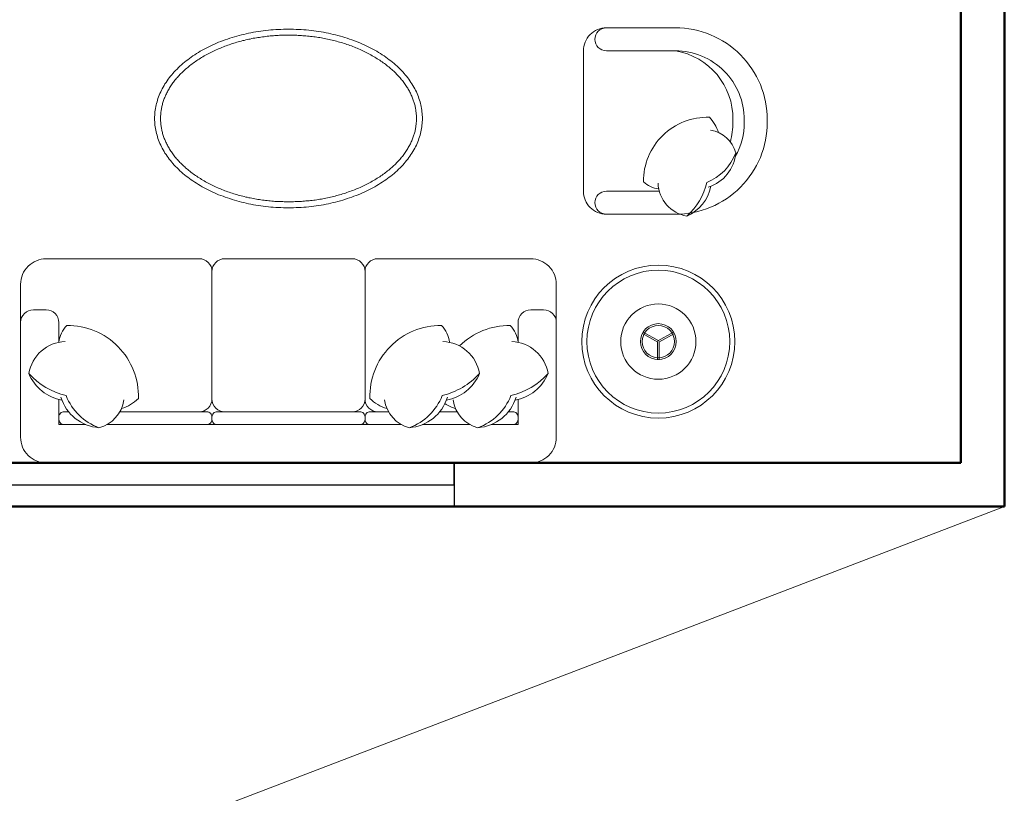
# Model space of a CAD drawing. Units: inches. Extents: x 1901 to 2863, y 888 to 2433.
# Tile 68 of 91: x 2651 to 2753, y 1732 to 1812. Entities that reach past the tile are written whole.
import ezdxf

# ---------------------------------------------------------------- set-up
doc = ezdxf.new("R2010")
doc.units = ezdxf.units.IN
for name, color, linetype, lineweight in [('A-ANNO-SYMB', 8, 'Continuous', 13), ('A-FURN', 8, 'Continuous', 18), ('A-GLAZ', 3, 'Continuous', 25), ('A-WALL', 7, 'Continuous', 50)]:
    doc.layers.add(name, color=color, linetype=linetype, lineweight=lineweight)

# ---------------------------------------------------------------- blocks, each defined once
blk = doc.blocks.new('WIN-60')
for p, q in [((0, 4.5), (0, 0)), ((60, 2.25), (60, 4.5)), ((60, 4.5), (60, 0)), ((0, 0), (0, 2.25)), ((0, 2.25), (60, 2.25))]:
    blk.add_line(p, q)

msp = doc.modelspace()

# ---------------------------------------------------------------- linework, layer by layer
at = {"layer": 'A-ANNO-SYMB'}
msp.add_line((2752.93, 1761.63), (2502.24, 1665.63), dxfattribs=at)
at = {"layer": 'A-FURN', "ltscale": 0.03}
for p, q in [((2717.24, 1778.55), (2715.64, 1779.47)), ((2717.32, 1778.69), (2715.72, 1779.61)), ((2717.24, 1778.69), (2718.85, 1779.61)), ((2717.32, 1778.55), (2718.93, 1779.47)), ((2717.2, 1778.62), (2717.2, 1776.76)), ((2717.36, 1778.62), (2717.36, 1776.76))]:
    msp.add_line(p, q, dxfattribs=at)
msp.add_lwpolyline([(2709.56, 1801.35), (2709.56, 1808.58, -0.414214), (2711.93, 1810.95), (2719.04, 1810.95, -0.414214), (2728.51, 1801.47), (2728.51, 1801.35), (2728.51, 1801.23, -0.414214), (2719.04, 1791.75), (2711.93, 1791.75, -0.414214), (2709.56, 1794.12), (2709.56, 1801.35)], format="xyb", dxfattribs=at)
at = {"layer": 'A-FURN'}
for points in [[(2719.04, 1808.58), (2711.93, 1808.58, -0.414214), (2710.74, 1809.76), (2710.74, 1809.76, -0.414214), (2711.93, 1810.95)], [(2719.04, 1808.58, -0.372719), (2724.96, 1801.47), (2724.96, 1801.35)], [(2719.04, 1808.58, -0.414214), (2726.14, 1801.47), (2726.14, 1801.35)], [(2717.32, 1794.36, -0.165541), (2715.75, 1795.09, -0.425989), (2722.54, 1801.74, -0.121523), (2723.47, 1800.16, 7.115464)], [(2724.7, 1799.21, 0.072384), (2724.96, 1801.23), (2724.96, 1801.35)], [(2725.21, 1797.7, 0.130591), (2726.14, 1801.23), (2726.14, 1801.35)], [(2722.43, 1794.54, 0.306663), (2725.25, 1798.08, 0.30633), (2722.67, 1800.39, -0.872847)], [(2720.23, 1791.56, 0.14773), (2722.27, 1795.02, 0.213343), (2725.25, 1798.08, 0.178662)], [(2717.25, 1794.95, 0.356772), (2720.23, 1791.56, 0.249542), (2722.69, 1794.63, -9.61688)], [(2717.37, 1794.12), (2711.93, 1794.12, 0.414214), (2710.74, 1792.94), (2710.74, 1792.94, 0.414214), (2711.93, 1791.75)], [(2669.98, 1771.39, 0.414214), (2671.29, 1772.7), (2671.29, 1785.84, 0.414214)], [(2688.37, 1771.39, -0.414214), (2687.06, 1772.7), (2687.06, 1785.84, -0.414214)], [(2651.58, 1780.59, -0.414214), (2652.9, 1781.9), (2654.21, 1781.9, -0.414214), (2655.52, 1780.59), (2655.52, 1778.55)], [(2702.83, 1778.55), (2702.83, 1780.59, -0.414214), (2704.14, 1781.9), (2705.46, 1781.9, -0.414214), (2706.77, 1780.59)], [(2655.52, 1778.55, -0.165541), (2656.33, 1780.29, -0.425989), (2663.71, 1772.76, -0.121523), (2661.96, 1771.72, 7.115464)], [(2695.75, 1778.55, 0.165541), (2694.94, 1780.29, 0.425989), (2687.56, 1772.76, 0.121523), (2689.31, 1771.72, -7.115464)], [(2702.83, 1778.55, 0.165541), (2702.02, 1780.29, 0.200231), (2696.8, 1778.17, 0.121523)], [(2656.18, 1778.63, 0.356772), (2652.42, 1775.32, 0.249542), (2655.83, 1772.59, -9.61688)], [(2695.09, 1778.63, -0.356772), (2698.86, 1775.32, -0.249542), (2695.44, 1772.59, 9.61688)], [(2702.17, 1778.63, -0.356772), (2705.93, 1775.32, -0.249542), (2702.52, 1772.59, 9.61688)], [(2652.42, 1775.32, 0.14773), (2656.26, 1773.06, 0.213343), (2659.65, 1769.75, 0.178662)], [(2698.86, 1775.32, -0.14773), (2695.01, 1773.06, -0.213343), (2691.63, 1769.75, -0.178662)], [(2705.93, 1775.32, -0.14773), (2702.09, 1773.06, -0.213343), (2698.7, 1769.75, -0.178662)], [(2655.73, 1772.88, 0.306663), (2659.65, 1769.75, 0.30633), (2662.21, 1772.61, -0.872847)], [(2672.61, 1771.39, -0.414214), (2671.29, 1772.7)], [(2685.75, 1771.39, 0.414214), (2687.06, 1772.7)], [(2695.55, 1772.88, -0.306663), (2691.63, 1769.75, -0.30633), (2689.07, 1772.61, 0.872847)], [(2702.62, 1772.88, -0.306663), (2698.7, 1769.75, -0.30633), (2696.14, 1772.61, 0.872847)], [(2700.06, 1770.08), (2702.83, 1770.08), (2702.83, 1772.66, -0.414214)], [(2656.53, 1771.39), (2656.05, 1771.39, 0.414214), (2655.52, 1770.86), (2655.52, 1770.6, 0.414214), (2656.05, 1770.08)], [(2660.47, 1770.08), (2670.77, 1770.08, 0.414214), (2671.29, 1770.6), (2671.29, 1770.86, 0.414214), (2670.77, 1771.39), (2661.8, 1771.39, 0.414214)], [(2690.8, 1770.08), (2687.59, 1770.08, -0.414214), (2687.06, 1770.6), (2687.06, 1770.86, -0.414214), (2687.59, 1771.39), (2689.48, 1771.39, -0.414214)], [(2694.75, 1771.39), (2696.55, 1771.39, -0.414214)], [(2695.29, 1772.24, 0.071865), (2696.39, 1771.72, -7.115464)], [(2701.83, 1771.39), (2702.3, 1771.39, -0.414214), (2702.83, 1770.86), (2702.83, 1770.6, -0.414214), (2702.3, 1770.08)], [(2656.05, 1770.08), (2658.29, 1770.08, 0.414214)], [(2697.88, 1770.08), (2692.99, 1770.08, -0.414214)], [(2702.3, 1770.08), (2700.06, 1770.08, -0.414214)]]:
    msp.add_lwpolyline(points, format="xyb", dxfattribs=at)
at = {"layer": 'A-FURN', "ltscale": 0.03}
msp.add_lwpolyline([(2651.58, 1784.53, -0.414214), (2654.21, 1787.16), (2669.98, 1787.16, -0.414214), (2671.29, 1785.84, -0.414214), (2672.61, 1787.16), (2685.75, 1787.16, -0.414214), (2687.06, 1785.84, -0.414214), (2688.37, 1787.16), (2704.14, 1787.16, -0.414214), (2706.77, 1784.53), (2706.77, 1768.76, -0.414214), (2704.14, 1766.13), (2654.21, 1766.13, -0.414214), (2651.58, 1768.76)], format="xyb", close=True, dxfattribs=at)
at = {"layer": 'A-FURN'}
for points in [[(2655.52, 1772.66), (2655.52, 1770.08), (2658.29, 1770.08)], [(2660.47, 1770.08), (2690.8, 1770.08)], [(2692.99, 1770.08), (2697.88, 1770.08)]]:
    msp.add_lwpolyline(points, dxfattribs=at)
msp.add_lwpolyline([(2686.53, 1770.08), (2671.82, 1770.08, -0.414214), (2671.29, 1770.6), (2671.29, 1770.86, -0.414214), (2671.82, 1771.39), (2686.53, 1771.39, -0.414214), (2687.06, 1770.86), (2687.06, 1770.6, -0.414214)], format="xyb", close=True, dxfattribs=at)
at = {"layer": 'A-FURN', "ltscale": 0.03}
msp.add_polyline3d([(2665.38, 1801.61, 0), (2665.38, 1801.44, 0), (2665.39, 1801.26, 0), (2665.4, 1801.09, 0), (2665.42, 1800.92, 0), (2665.44, 1800.74, 0), (2665.47, 1800.57, 0), (2665.5, 1800.4, 0), (2665.54, 1800.22, 0), (2665.58, 1800.05, 0), (2665.63, 1799.88, 0), (2665.68, 1799.71, 0), (2665.73, 1799.54, 0), (2665.79, 1799.37, 0), (2665.86, 1799.2, 0), (2665.93, 1799.04, 0), (2666.01, 1798.87, 0), (2666.09, 1798.7, 0), (2666.17, 1798.54, 0), (2666.26, 1798.38, 0), (2666.36, 1798.21, 0), (2666.45, 1798.05, 0), (2666.56, 1797.89, 0), (2666.67, 1797.73, 0), (2666.78, 1797.58, 0), (2666.89, 1797.42, 0), (2667.02, 1797.27, 0), (2667.14, 1797.11, 0), (2667.27, 1796.96, 0), (2667.41, 1796.81, 0), (2667.54, 1796.67, 0), (2667.69, 1796.52, 0), (2667.83, 1796.38, 0), (2667.98, 1796.23, 0), (2668.14, 1796.09, 0), (2668.3, 1795.95, 0), (2668.46, 1795.82, 0), (2668.63, 1795.68, 0), (2668.8, 1795.55, 0), (2668.97, 1795.42, 0), (2669.15, 1795.3, 0), (2669.33, 1795.17, 0), (2669.51, 1795.05, 0), (2669.7, 1794.93, 0), (2669.89, 1794.81, 0), (2670.09, 1794.69, 0), (2670.29, 1794.58, 0), (2670.49, 1794.47, 0), (2670.69, 1794.36, 0), (2670.9, 1794.25, 0), (2671.11, 1794.15, 0), (2671.32, 1794.05, 0), (2671.54, 1793.95, 0), (2671.76, 1793.86, 0), (2671.98, 1793.76, 0), (2672.2, 1793.68, 0), (2672.43, 1793.59, 0), (2672.66, 1793.5, 0), (2672.89, 1793.42, 0), (2673.12, 1793.35, 0), (2673.36, 1793.27, 0), (2673.6, 1793.2, 0), (2673.84, 1793.13, 0), (2674.08, 1793.06, 0), (2674.32, 1793, 0), (2674.57, 1792.94, 0), (2674.81, 1792.89, 0), (2675.06, 1792.83, 0), (2675.31, 1792.78, 0), (2675.56, 1792.73, 0), (2675.82, 1792.69, 0), (2676.07, 1792.65, 0), (2676.32, 1792.61, 0), (2676.58, 1792.58, 0), (2676.84, 1792.55, 0), (2677.1, 1792.52, 0), (2677.35, 1792.49, 0), (2677.61, 1792.47, 0), (2677.87, 1792.45, 0), (2678.13, 1792.44, 0), (2678.39, 1792.43, 0), (2678.65, 1792.42, 0), (2678.92, 1792.42, 0), (2679.18, 1792.41, 0), (2679.44, 1792.42, 0), (2679.7, 1792.42, 0), (2679.96, 1792.43, 0), (2680.22, 1792.44, 0), (2680.48, 1792.45, 0), (2680.74, 1792.47, 0), (2681, 1792.49, 0), (2681.26, 1792.52, 0), (2681.51, 1792.55, 0), (2681.77, 1792.58, 0), (2682.03, 1792.61, 0), (2682.28, 1792.65, 0), (2682.54, 1792.69, 0), (2682.79, 1792.73, 0), (2683.04, 1792.78, 0), (2683.29, 1792.83, 0), (2683.54, 1792.89, 0), (2683.79, 1792.94, 0), (2684.03, 1793, 0), (2684.27, 1793.06, 0), (2684.52, 1793.13, 0), (2684.76, 1793.2, 0), (2684.99, 1793.27, 0), (2685.23, 1793.35, 0), (2685.46, 1793.42, 0), (2685.69, 1793.5, 0), (2685.92, 1793.59, 0), (2686.15, 1793.68, 0), (2686.37, 1793.76, 0), (2686.6, 1793.86, 0), (2686.81, 1793.95, 0), (2687.03, 1794.05, 0), (2687.24, 1794.15, 0), (2687.45, 1794.25, 0), (2687.66, 1794.36, 0), (2687.87, 1794.47, 0), (2688.07, 1794.58, 0), (2688.26, 1794.69, 0), (2688.46, 1794.81, 0), (2688.65, 1794.93, 0), (2688.84, 1795.05, 0), (2689.02, 1795.17, 0), (2689.21, 1795.3, 0), (2689.38, 1795.42, 0), (2689.56, 1795.55, 0), (2689.73, 1795.68, 0), (2689.89, 1795.82, 0), (2690.06, 1795.95, 0), (2690.21, 1796.09, 0), (2690.37, 1796.23, 0), (2690.52, 1796.38, 0), (2690.67, 1796.52, 0), (2690.81, 1796.67, 0), (2690.95, 1796.81, 0), (2691.08, 1796.96, 0), (2691.21, 1797.11, 0), (2691.34, 1797.27, 0), (2691.46, 1797.42, 0), (2691.57, 1797.58, 0), (2691.69, 1797.73, 0), (2691.79, 1797.89, 0), (2691.9, 1798.05, 0), (2692, 1798.21, 0), (2692.09, 1798.38, 0), (2692.18, 1798.54, 0), (2692.27, 1798.7, 0), (2692.35, 1798.87, 0), (2692.42, 1799.04, 0), (2692.49, 1799.2, 0), (2692.56, 1799.37, 0), (2692.62, 1799.54, 0), (2692.68, 1799.71, 0), (2692.73, 1799.88, 0), (2692.77, 1800.05, 0), (2692.82, 1800.22, 0), (2692.85, 1800.4, 0), (2692.88, 1800.57, 0), (2692.91, 1800.74, 0), (2692.93, 1800.92, 0), (2692.95, 1801.09, 0), (2692.96, 1801.26, 0), (2692.97, 1801.44, 0), (2692.97, 1801.61, 0), (2692.97, 1801.79, 0), (2692.96, 1801.96, 0), (2692.95, 1802.13, 0), (2692.93, 1802.31, 0), (2692.91, 1802.48, 0), (2692.88, 1802.65, 0), (2692.85, 1802.83, 0), (2692.82, 1803, 0), (2692.77, 1803.17, 0), (2692.73, 1803.34, 0), (2692.68, 1803.51, 0), (2692.62, 1803.68, 0), (2692.56, 1803.85, 0), (2692.49, 1804.02, 0), (2692.42, 1804.19, 0), (2692.35, 1804.35, 0), (2692.27, 1804.52, 0), (2692.18, 1804.68, 0), (2692.09, 1804.85, 0), (2692, 1805.01, 0), (2691.9, 1805.17, 0), (2691.79, 1805.33, 0), (2691.69, 1805.49, 0), (2691.57, 1805.65, 0), (2691.46, 1805.8, 0), (2691.34, 1805.96, 0), (2691.21, 1806.11, 0), (2691.08, 1806.26, 0), (2690.95, 1806.41, 0), (2690.81, 1806.56, 0), (2690.67, 1806.7, 0), (2690.52, 1806.85, 0), (2690.37, 1806.99, 0), (2690.21, 1807.13, 0), (2690.06, 1807.27, 0), (2689.89, 1807.4, 0), (2689.73, 1807.54, 0), (2689.56, 1807.67, 0), (2689.38, 1807.8, 0), (2689.21, 1807.93, 0), (2689.02, 1808.05, 0), (2688.84, 1808.18, 0), (2688.65, 1808.3, 0), (2688.46, 1808.42, 0), (2688.26, 1808.53, 0), (2688.07, 1808.65, 0), (2687.87, 1808.76, 0), (2687.66, 1808.86, 0), (2687.45, 1808.97, 0), (2687.24, 1809.07, 0), (2687.03, 1809.17, 0), (2686.81, 1809.27, 0), (2686.6, 1809.37, 0), (2686.37, 1809.46, 0), (2686.15, 1809.55, 0), (2685.92, 1809.63, 0), (2685.69, 1809.72, 0), (2685.46, 1809.8, 0), (2685.23, 1809.88, 0), (2684.99, 1809.95, 0), (2684.76, 1810.02, 0), (2684.52, 1810.09, 0), (2684.27, 1810.16, 0), (2684.03, 1810.22, 0), (2683.79, 1810.28, 0), (2683.54, 1810.34, 0), (2683.29, 1810.39, 0), (2683.04, 1810.44, 0), (2682.79, 1810.49, 0), (2682.54, 1810.53, 0), (2682.28, 1810.57, 0), (2682.03, 1810.61, 0), (2681.77, 1810.65, 0), (2681.51, 1810.68, 0), (2681.26, 1810.7, 0), (2681, 1810.73, 0), (2680.74, 1810.75, 0), (2680.48, 1810.77, 0), (2680.22, 1810.78, 0), (2679.96, 1810.79, 0), (2679.7, 1810.8, 0), (2679.44, 1810.81, 0), (2679.18, 1810.81, 0), (2678.92, 1810.81, 0), (2678.65, 1810.8, 0), (2678.39, 1810.79, 0), (2678.13, 1810.78, 0), (2677.87, 1810.77, 0), (2677.61, 1810.75, 0), (2677.35, 1810.73, 0), (2677.1, 1810.7, 0), (2676.84, 1810.68, 0), (2676.58, 1810.65, 0), (2676.32, 1810.61, 0), (2676.07, 1810.57, 0), (2675.82, 1810.53, 0), (2675.56, 1810.49, 0), (2675.31, 1810.44, 0), (2675.06, 1810.39, 0), (2674.81, 1810.34, 0), (2674.57, 1810.28, 0), (2674.32, 1810.22, 0), (2674.08, 1810.16, 0), (2673.84, 1810.09, 0), (2673.6, 1810.02, 0), (2673.36, 1809.95, 0), (2673.12, 1809.88, 0), (2672.89, 1809.8, 0), (2672.66, 1809.72, 0), (2672.43, 1809.63, 0), (2672.2, 1809.55, 0), (2671.98, 1809.46, 0), (2671.76, 1809.37, 0), (2671.54, 1809.27, 0), (2671.32, 1809.17, 0), (2671.11, 1809.07, 0), (2670.9, 1808.97, 0), (2670.69, 1808.86, 0), (2670.49, 1808.76, 0), (2670.29, 1808.65, 0), (2670.09, 1808.53, 0), (2669.89, 1808.42, 0), (2669.7, 1808.3, 0), (2669.51, 1808.18, 0), (2669.33, 1808.05, 0), (2669.15, 1807.93, 0), (2668.97, 1807.8, 0), (2668.8, 1807.67, 0), (2668.63, 1807.54, 0), (2668.46, 1807.4, 0), (2668.3, 1807.27, 0), (2668.14, 1807.13, 0), (2667.98, 1806.99, 0), (2667.83, 1806.85, 0), (2667.69, 1806.7, 0), (2667.54, 1806.56, 0), (2667.41, 1806.41, 0), (2667.27, 1806.26, 0), (2667.14, 1806.11, 0), (2667.02, 1805.96, 0), (2666.89, 1805.8, 0), (2666.78, 1805.65, 0), (2666.67, 1805.49, 0), (2666.56, 1805.33, 0), (2666.45, 1805.17, 0), (2666.36, 1805.01, 0), (2666.26, 1804.85, 0), (2666.17, 1804.68, 0), (2666.09, 1804.52, 0), (2666.01, 1804.35, 0), (2665.93, 1804.19, 0), (2665.86, 1804.02, 0), (2665.79, 1803.85, 0), (2665.73, 1803.68, 0), (2665.68, 1803.51, 0), (2665.63, 1803.34, 0), (2665.58, 1803.17, 0), (2665.54, 1803, 0), (2665.5, 1802.83, 0), (2665.47, 1802.65, 0), (2665.44, 1802.48, 0), (2665.42, 1802.31, 0), (2665.4, 1802.13, 0), (2665.39, 1801.96, 0), (2665.38, 1801.79, 0), (2665.38, 1801.61, 0)], dxfattribs=at)
at = {"layer": 'A-FURN'}
msp.add_polyline3d([(2665.99, 1801.61, 0), (2665.99, 1801.52, 0), (2666, 1801.42, 0), (2666, 1801.33, 0), (2666.01, 1801.23, 0), (2666.01, 1801.14, 0), (2666.02, 1801.04, 0), (2666.03, 1800.94, 0), (2666.05, 1800.85, 0), (2666.06, 1800.75, 0), (2666.08, 1800.65, 0), (2666.09, 1800.56, 0), (2666.11, 1800.46, 0), (2666.14, 1800.36, 0), (2666.16, 1800.26, 0), (2666.18, 1800.16, 0), (2666.21, 1800.06, 0), (2666.24, 1799.96, 0), (2666.27, 1799.86, 0), (2666.31, 1799.76, 0), (2666.34, 1799.66, 0), (2666.38, 1799.56, 0), (2666.42, 1799.46, 0), (2666.46, 1799.36, 0), (2666.5, 1799.26, 0), (2666.55, 1799.16, 0), (2666.6, 1799.06, 0), (2666.65, 1798.96, 0), (2666.7, 1798.86, 0), (2666.75, 1798.76, 0), (2666.81, 1798.66, 0), (2666.87, 1798.56, 0), (2666.93, 1798.46, 0), (2666.99, 1798.36, 0), (2667.05, 1798.26, 0), (2667.12, 1798.16, 0), (2667.19, 1798.06, 0), (2667.26, 1797.96, 0), (2667.33, 1797.86, 0), (2667.41, 1797.76, 0), (2667.48, 1797.66, 0), (2667.56, 1797.56, 0), (2667.65, 1797.47, 0), (2667.73, 1797.37, 0), (2667.82, 1797.27, 0), (2667.9, 1797.18, 0), (2667.99, 1797.08, 0), (2668.09, 1796.99, 0), (2668.18, 1796.9, 0), (2668.28, 1796.8, 0), (2668.38, 1796.71, 0), (2668.48, 1796.62, 0), (2668.58, 1796.53, 0), (2668.69, 1796.43, 0), (2668.8, 1796.34, 0), (2668.9, 1796.26, 0), (2669.02, 1796.17, 0), (2669.13, 1796.08, 0), (2669.24, 1795.99, 0), (2669.36, 1795.91, 0), (2669.48, 1795.82, 0), (2669.6, 1795.74, 0), (2669.72, 1795.66, 0), (2669.84, 1795.57, 0), (2669.97, 1795.49, 0), (2670.1, 1795.41, 0), (2670.22, 1795.33, 0), (2670.35, 1795.25, 0), (2670.49, 1795.18, 0), (2670.62, 1795.1, 0), (2670.75, 1795.03, 0), (2670.89, 1794.95, 0), (2671.03, 1794.88, 0), (2671.16, 1794.81, 0), (2671.3, 1794.74, 0), (2671.45, 1794.67, 0), (2671.59, 1794.6, 0), (2671.73, 1794.54, 0), (2671.88, 1794.47, 0), (2672.02, 1794.41, 0), (2672.17, 1794.35, 0), (2672.32, 1794.29, 0), (2672.47, 1794.23, 0), (2672.62, 1794.17, 0), (2672.77, 1794.12, 0), (2672.92, 1794.06, 0), (2673.07, 1794.01, 0), (2673.23, 1793.96, 0), (2673.38, 1793.91, 0), (2673.53, 1793.86, 0), (2673.69, 1793.81, 0), (2673.84, 1793.77, 0), (2673.99, 1793.72, 0), (2674.15, 1793.68, 0), (2674.3, 1793.64, 0), (2674.46, 1793.6, 0), (2674.61, 1793.56, 0), (2674.77, 1793.52, 0), (2674.93, 1793.49, 0), (2675.08, 1793.45, 0), (2675.24, 1793.42, 0), (2675.4, 1793.39, 0), (2675.55, 1793.36, 0), (2675.71, 1793.33, 0), (2675.87, 1793.3, 0), (2676.03, 1793.27, 0), (2676.19, 1793.25, 0), (2676.34, 1793.23, 0), (2676.5, 1793.2, 0), (2676.66, 1793.18, 0), (2676.82, 1793.16, 0), (2676.98, 1793.15, 0), (2677.14, 1793.13, 0), (2677.3, 1793.11, 0), (2677.46, 1793.1, 0), (2677.62, 1793.09, 0), (2677.78, 1793.07, 0), (2677.94, 1793.06, 0), (2678.1, 1793.06, 0), (2678.26, 1793.05, 0), (2678.42, 1793.04, 0), (2678.58, 1793.04, 0), (2678.74, 1793.03, 0), (2678.9, 1793.03, 0), (2679.06, 1793.03, 0), (2679.22, 1793.03, 0), (2679.38, 1793.03, 0), (2679.54, 1793.03, 0), (2679.7, 1793.03, 0), (2679.86, 1793.04, 0), (2680.02, 1793.04, 0), (2680.18, 1793.05, 0), (2680.34, 1793.06, 0), (2680.5, 1793.07, 0), (2680.66, 1793.08, 0), (2680.82, 1793.09, 0), (2680.97, 1793.11, 0), (2681.13, 1793.12, 0), (2681.29, 1793.14, 0), (2681.45, 1793.15, 0), (2681.61, 1793.17, 0), (2681.77, 1793.19, 0), (2681.93, 1793.21, 0), (2682.09, 1793.24, 0), (2682.25, 1793.26, 0), (2682.4, 1793.29, 0), (2682.56, 1793.31, 0), (2682.72, 1793.34, 0), (2682.88, 1793.37, 0), (2683.03, 1793.4, 0), (2683.19, 1793.43, 0), (2683.35, 1793.47, 0), (2683.5, 1793.5, 0), (2683.66, 1793.54, 0), (2683.82, 1793.58, 0), (2683.97, 1793.62, 0), (2684.13, 1793.66, 0), (2684.28, 1793.7, 0), (2684.44, 1793.74, 0), (2684.59, 1793.79, 0), (2684.74, 1793.84, 0), (2684.9, 1793.88, 0), (2685.05, 1793.93, 0), (2685.2, 1793.98, 0), (2685.36, 1794.04, 0), (2685.51, 1794.09, 0), (2685.66, 1794.14, 0), (2685.81, 1794.2, 0), (2685.96, 1794.26, 0), (2686.11, 1794.32, 0), (2686.26, 1794.38, 0), (2686.4, 1794.44, 0), (2686.55, 1794.51, 0), (2686.69, 1794.57, 0), (2686.84, 1794.64, 0), (2686.98, 1794.71, 0), (2687.12, 1794.78, 0), (2687.26, 1794.85, 0), (2687.39, 1794.92, 0), (2687.53, 1794.99, 0), (2687.67, 1795.06, 0), (2687.8, 1795.14, 0), (2687.93, 1795.22, 0), (2688.06, 1795.29, 0), (2688.19, 1795.37, 0), (2688.32, 1795.45, 0), (2688.45, 1795.53, 0), (2688.57, 1795.61, 0), (2688.69, 1795.7, 0), (2688.81, 1795.78, 0), (2688.93, 1795.86, 0), (2689.05, 1795.95, 0), (2689.17, 1796.04, 0), (2689.28, 1796.12, 0), (2689.39, 1796.21, 0), (2689.5, 1796.3, 0), (2689.61, 1796.39, 0), (2689.72, 1796.48, 0), (2689.82, 1796.57, 0), (2689.92, 1796.66, 0), (2690.02, 1796.76, 0), (2690.12, 1796.85, 0), (2690.22, 1796.94, 0), (2690.31, 1797.04, 0), (2690.4, 1797.13, 0), (2690.49, 1797.23, 0), (2690.58, 1797.32, 0), (2690.67, 1797.42, 0), (2690.75, 1797.52, 0), (2690.83, 1797.61, 0), (2690.91, 1797.71, 0), (2690.98, 1797.81, 0), (2691.06, 1797.91, 0), (2691.13, 1798.01, 0), (2691.2, 1798.11, 0), (2691.27, 1798.21, 0), (2691.33, 1798.31, 0), (2691.4, 1798.41, 0), (2691.46, 1798.51, 0), (2691.52, 1798.61, 0), (2691.57, 1798.71, 0), (2691.63, 1798.81, 0), (2691.68, 1798.91, 0), (2691.73, 1799.01, 0), (2691.78, 1799.11, 0), (2691.83, 1799.21, 0), (2691.87, 1799.31, 0), (2691.91, 1799.41, 0), (2691.95, 1799.51, 0), (2691.99, 1799.61, 0), (2692.03, 1799.71, 0), (2692.06, 1799.81, 0), (2692.1, 1799.91, 0), (2692.13, 1800.01, 0), (2692.15, 1800.11, 0), (2692.18, 1800.21, 0), (2692.21, 1800.31, 0), (2692.23, 1800.41, 0), (2692.25, 1800.51, 0), (2692.27, 1800.6, 0), (2692.28, 1800.7, 0), (2692.3, 1800.8, 0), (2692.31, 1800.9, 0), (2692.33, 1800.99, 0), (2692.34, 1801.09, 0), (2692.34, 1801.19, 0), (2692.35, 1801.28, 0), (2692.35, 1801.38, 0), (2692.36, 1801.47, 0), (2692.36, 1801.56, 0), (2692.36, 1801.66, 0), (2692.36, 1801.75, 0), (2692.35, 1801.85, 0), (2692.35, 1801.94, 0), (2692.34, 1802.04, 0), (2692.34, 1802.13, 0), (2692.33, 1802.23, 0), (2692.31, 1802.33, 0), (2692.3, 1802.42, 0), (2692.28, 1802.52, 0), (2692.27, 1802.62, 0), (2692.25, 1802.72, 0), (2692.23, 1802.82, 0), (2692.21, 1802.91, 0), (2692.18, 1803.01, 0), (2692.15, 1803.11, 0), (2692.13, 1803.21, 0), (2692.1, 1803.31, 0), (2692.06, 1803.41, 0), (2692.03, 1803.51, 0), (2691.99, 1803.61, 0), (2691.95, 1803.71, 0), (2691.91, 1803.81, 0), (2691.87, 1803.91, 0), (2691.83, 1804.01, 0), (2691.78, 1804.11, 0), (2691.73, 1804.21, 0), (2691.68, 1804.31, 0), (2691.63, 1804.42, 0), (2691.57, 1804.52, 0), (2691.52, 1804.62, 0), (2691.46, 1804.72, 0), (2691.4, 1804.82, 0), (2691.33, 1804.92, 0), (2691.27, 1805.02, 0), (2691.2, 1805.12, 0), (2691.13, 1805.22, 0), (2691.06, 1805.31, 0), (2690.98, 1805.41, 0), (2690.91, 1805.51, 0), (2690.83, 1805.61, 0), (2690.75, 1805.71, 0), (2690.67, 1805.8, 0), (2690.58, 1805.9, 0), (2690.49, 1806, 0), (2690.4, 1806.09, 0), (2690.31, 1806.19, 0), (2690.22, 1806.28, 0), (2690.12, 1806.38, 0), (2690.02, 1806.47, 0), (2689.92, 1806.56, 0), (2689.82, 1806.65, 0), (2689.72, 1806.74, 0), (2689.61, 1806.83, 0), (2689.5, 1806.92, 0), (2689.39, 1807.01, 0), (2689.28, 1807.1, 0), (2689.17, 1807.19, 0), (2689.05, 1807.27, 0), (2688.93, 1807.36, 0), (2688.81, 1807.44, 0), (2688.69, 1807.53, 0), (2688.57, 1807.61, 0), (2688.45, 1807.69, 0), (2688.32, 1807.77, 0), (2688.19, 1807.85, 0), (2688.06, 1807.93, 0), (2687.93, 1808.01, 0), (2687.8, 1808.08, 0), (2687.67, 1808.16, 0), (2687.53, 1808.23, 0), (2687.39, 1808.31, 0), (2687.26, 1808.38, 0), (2687.12, 1808.45, 0), (2686.98, 1808.52, 0), (2686.84, 1808.59, 0), (2686.69, 1808.65, 0), (2686.55, 1808.72, 0), (2686.4, 1808.78, 0), (2686.26, 1808.84, 0), (2686.11, 1808.9, 0), (2685.96, 1808.96, 0), (2685.81, 1809.02, 0), (2685.66, 1809.08, 0), (2685.51, 1809.13, 0), (2685.36, 1809.19, 0), (2685.2, 1809.24, 0), (2685.05, 1809.29, 0), (2684.9, 1809.34, 0), (2684.74, 1809.39, 0), (2684.59, 1809.43, 0), (2684.44, 1809.48, 0), (2684.28, 1809.52, 0), (2684.13, 1809.57, 0), (2683.97, 1809.61, 0), (2683.82, 1809.65, 0), (2683.66, 1809.68, 0), (2683.5, 1809.72, 0), (2683.35, 1809.75, 0), (2683.19, 1809.79, 0), (2683.03, 1809.82, 0), (2682.88, 1809.85, 0), (2682.72, 1809.88, 0), (2682.56, 1809.91, 0), (2682.4, 1809.94, 0), (2682.25, 1809.96, 0), (2682.09, 1809.99, 0), (2681.93, 1810.01, 0), (2681.77, 1810.03, 0), (2681.61, 1810.05, 0), (2681.45, 1810.07, 0), (2681.29, 1810.09, 0), (2681.13, 1810.1, 0), (2680.97, 1810.12, 0), (2680.82, 1810.13, 0), (2680.66, 1810.14, 0), (2680.5, 1810.15, 0), (2680.34, 1810.16, 0), (2680.18, 1810.17, 0), (2680.02, 1810.18, 0), (2679.86, 1810.19, 0), (2679.7, 1810.19, 0), (2679.54, 1810.19, 0), (2679.38, 1810.2, 0), (2679.22, 1810.2, 0), (2679.06, 1810.2, 0), (2678.9, 1810.19, 0), (2678.74, 1810.19, 0), (2678.58, 1810.19, 0), (2678.42, 1810.18, 0), (2678.26, 1810.18, 0), (2678.1, 1810.17, 0), (2677.94, 1810.16, 0), (2677.78, 1810.15, 0), (2677.62, 1810.14, 0), (2677.46, 1810.12, 0), (2677.3, 1810.11, 0), (2677.14, 1810.09, 0), (2676.98, 1810.08, 0), (2676.82, 1810.06, 0), (2676.66, 1810.04, 0), (2676.5, 1810.02, 0), (2676.34, 1810, 0), (2676.19, 1809.97, 0), (2676.03, 1809.95, 0), (2675.87, 1809.92, 0), (2675.71, 1809.9, 0), (2675.55, 1809.87, 0), (2675.4, 1809.84, 0), (2675.24, 1809.8, 0), (2675.08, 1809.77, 0), (2674.93, 1809.74, 0), (2674.77, 1809.7, 0), (2674.61, 1809.66, 0), (2674.46, 1809.63, 0), (2674.3, 1809.59, 0), (2674.15, 1809.54, 0), (2673.99, 1809.5, 0), (2673.84, 1809.46, 0), (2673.69, 1809.41, 0), (2673.53, 1809.36, 0), (2673.38, 1809.32, 0), (2673.23, 1809.27, 0), (2673.07, 1809.21, 0), (2672.92, 1809.16, 0), (2672.77, 1809.11, 0), (2672.62, 1809.05, 0), (2672.47, 1808.99, 0), (2672.32, 1808.93, 0), (2672.17, 1808.87, 0), (2672.02, 1808.81, 0), (2671.88, 1808.75, 0), (2671.73, 1808.68, 0), (2671.59, 1808.62, 0), (2671.45, 1808.55, 0), (2671.3, 1808.48, 0), (2671.16, 1808.41, 0), (2671.03, 1808.34, 0), (2670.89, 1808.27, 0), (2670.75, 1808.2, 0), (2670.62, 1808.12, 0), (2670.49, 1808.05, 0), (2670.35, 1807.97, 0), (2670.22, 1807.89, 0), (2670.1, 1807.81, 0), (2669.97, 1807.73, 0), (2669.84, 1807.65, 0), (2669.72, 1807.57, 0), (2669.6, 1807.49, 0), (2669.48, 1807.4, 0), (2669.36, 1807.32, 0), (2669.24, 1807.23, 0), (2669.13, 1807.14, 0), (2669.02, 1807.06, 0), (2668.9, 1806.97, 0), (2668.8, 1806.88, 0), (2668.69, 1806.79, 0), (2668.58, 1806.7, 0), (2668.48, 1806.61, 0), (2668.38, 1806.51, 0), (2668.28, 1806.42, 0), (2668.18, 1806.33, 0), (2668.09, 1806.23, 0), (2667.99, 1806.14, 0), (2667.9, 1806.04, 0), (2667.82, 1805.95, 0), (2667.73, 1805.85, 0), (2667.65, 1805.76, 0), (2667.56, 1805.66, 0), (2667.48, 1805.56, 0), (2667.41, 1805.46, 0), (2667.33, 1805.36, 0), (2667.26, 1805.27, 0), (2667.19, 1805.17, 0), (2667.12, 1805.07, 0), (2667.05, 1804.97, 0), (2666.99, 1804.87, 0), (2666.93, 1804.77, 0), (2666.87, 1804.67, 0), (2666.81, 1804.57, 0), (2666.75, 1804.47, 0), (2666.7, 1804.37, 0), (2666.65, 1804.26, 0), (2666.6, 1804.16, 0), (2666.55, 1804.06, 0), (2666.5, 1803.96, 0), (2666.46, 1803.86, 0), (2666.42, 1803.76, 0), (2666.38, 1803.66, 0), (2666.34, 1803.56, 0), (2666.31, 1803.46, 0), (2666.27, 1803.36, 0), (2666.24, 1803.26, 0), (2666.21, 1803.16, 0), (2666.18, 1803.06, 0), (2666.16, 1802.96, 0), (2666.14, 1802.86, 0), (2666.11, 1802.77, 0), (2666.09, 1802.67, 0), (2666.08, 1802.57, 0), (2666.06, 1802.47, 0), (2666.05, 1802.38, 0), (2666.03, 1802.28, 0), (2666.02, 1802.18, 0), (2666.01, 1802.09, 0), (2666.01, 1801.99, 0), (2666, 1801.9, 0), (2666, 1801.8, 0), (2665.99, 1801.71, 0), (2665.99, 1801.61, 0)], dxfattribs=at)
at = {"layer": 'A-FURN', "ltscale": 0.03}
for radius in [7.88, 3.88, 1.85, 1.66]:
    msp.add_circle((2717.28, 1778.62), radius, dxfattribs=at)
at = {"layer": 'A-FURN'}
msp.add_circle((2717.28, 1778.62), 7.36, dxfattribs=at)
at = {"layer": 'A-WALL'}
for p, q in [((2748.43, 1817.13), (2748.43, 1766.13)), ((2752.93, 1761.63), (2752.93, 1812.63)), ((2748.43, 1766.13), (2609.93, 1766.13)), ((2482.11, 1761.63), (2752.93, 1761.63))]:
    msp.add_line(p, q, dxfattribs=at)

# ---------------------------------------------------------------- block references
at = {"layer": 'A-GLAZ'}
msp.add_blockref('WIN-60', (2636.23, 1761.63), dxfattribs=at)

doc.saveas('drawing.dxf')
